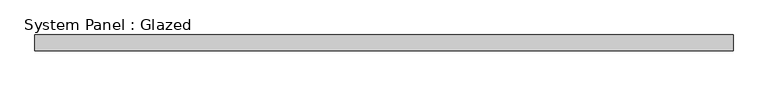
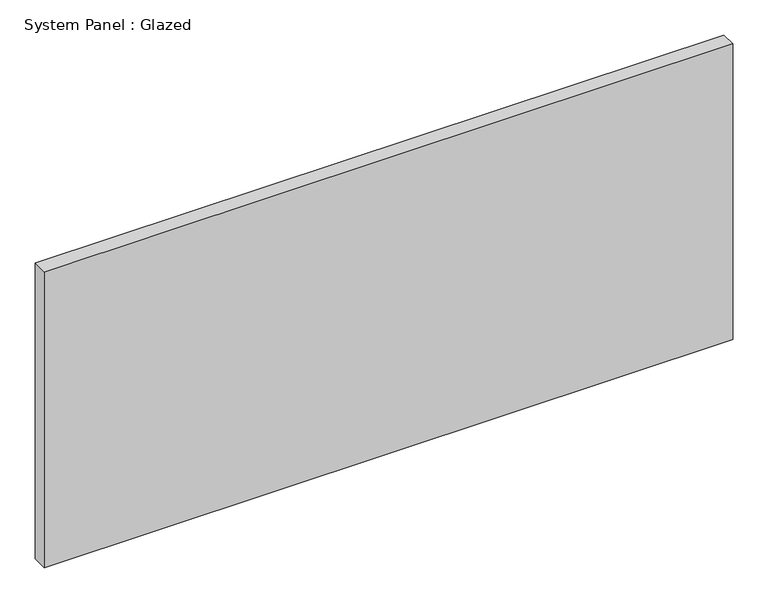
"""IFC4 building model written with IfcOpenShell, lengths in millimetres: plate geometry, System Panel : Glazed."""

from ifc_helpers import new_model, si_unit, origin, origin_with_axes, place, context, project, spatial, polyline, outline, extrude, source, transform, mapped, element, save


def system_panel_glazed_c20df1b6(model_context):
    return source(origin(), model_context, "Body", "SweptSolid", [
        extrude(outline(polyline([(566.2083333, 19.05), (-566.2083333, 19.05), (-566.2083333, 44.45), (566.2083333, 44.45), (566.2083333, 19.05)])), origin_with_axes(), (0.0, 0.0, 1.0), 514.35),
    ])


if __name__ == "__main__":
    model = new_model("IFC4")
    model_context = context("Model", 3, world=origin())
    ifc_project = project(units=[si_unit("LENGTHUNIT", "METRE", prefix="MILLI")], contexts=[model_context])
    site = spatial("IfcSite", under=ifc_project)
    building = spatial("IfcBuilding", under=site)
    placement = place(None, origin())
    system_panel_glazed_shape = system_panel_glazed_c20df1b6(model_context)
    element("IfcPlate", 1, ObjectType="System Panel : Glazed", at=placement, inside=building, context=model_context, shape_type="MappedRepresentation", body=[
        mapped(system_panel_glazed_shape, transform((0.0, 0.0, 0.0), x_axis=(1.0, 0.0, 0.0), y_axis=(0.0, 1.0, 0.0), z_axis=(0.0, 0.0, 1.0))),
    ])
    save(model, "model.ifc")

# Revit data of these elements
# Type "System Panel : Glazed"
#   Construction Type Id = "GSP4R"
#   Analytic Construction = "1/8 in Pilkington single glazing"
#   Visual Light Transmittance = 0.9
#   Solar Heat Gain Coefficient = 0.86
#   Heat Transfer Coefficient (U) = 1.18115 BTU/(h·ft²·°F)
# Element 1 (IfcPlate, "System Panel : Glazed")
#   Materials on its faces: "Glass"
# Materials
#   "Glass": class "Glass", colour RGB 0 128 192, transparency 0.75, Description = "Soda Lime Glass", Cost = 0
